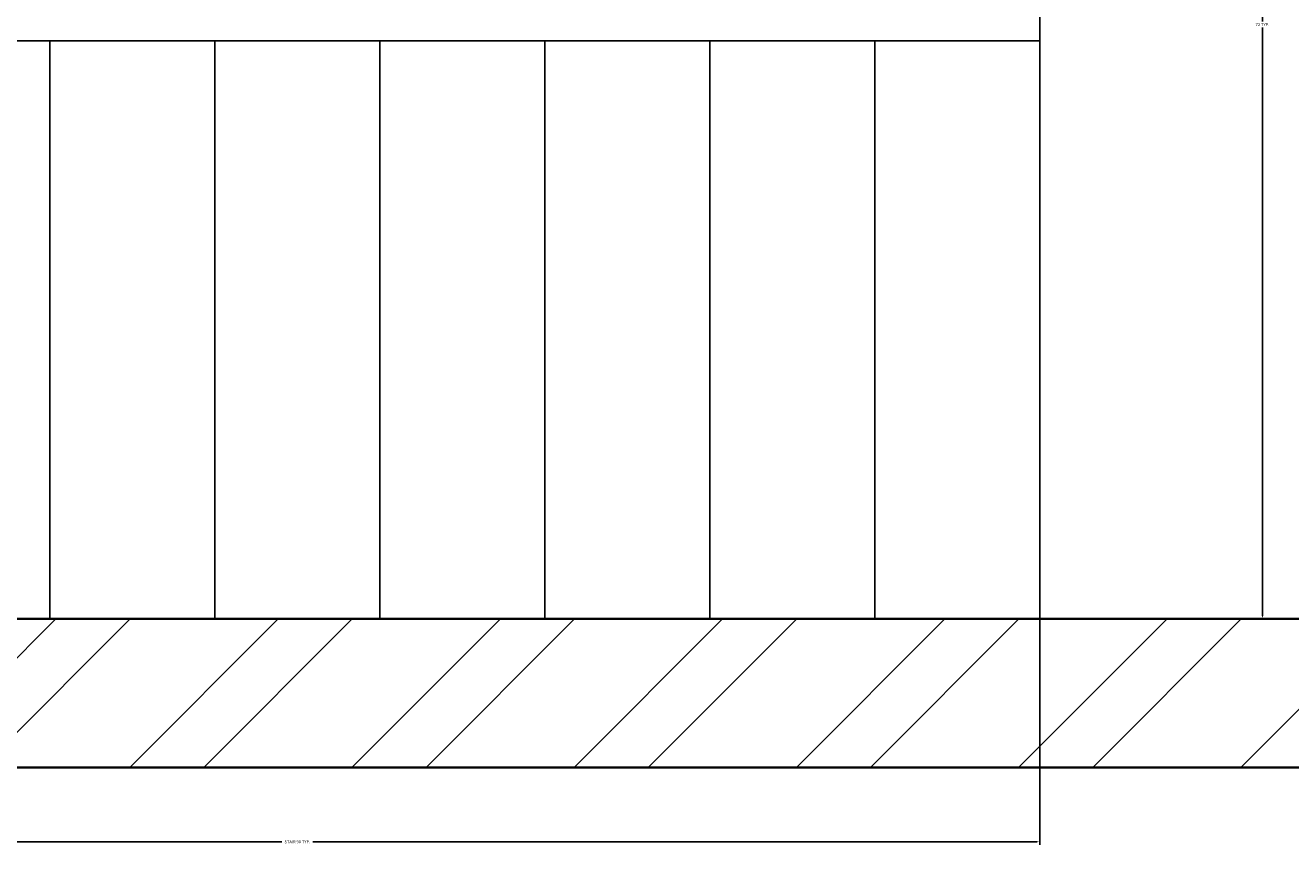
# Model space of a CAD drawing. Units: inches. Extents: x 2166 to 3588, y 1959 to 2628.
# Tile 9 of 13: x 3457 to 3534, y 2017 to 2067. Entities that reach past the tile are written whole.
import ezdxf

# ---------------------------------------------------------------- set-up
doc = ezdxf.new("R2010")
doc.units = ezdxf.units.IN
for name, color, linetype, lineweight in [('A-ANNO-DIMS', 2, 'Continuous', 18), ('A-AREA-IDEN', 170, 'Continuous', 18), ('A-WALL-PATT', 20, 'Continuous', 13), ('Staircase', 136, 'Continuous', 25), ('WALL', 40, 'Continuous', 35)]:
    doc.layers.add(name, color=color, linetype=linetype, lineweight=lineweight)
doc.styles.get("Standard").update_dxf_attribs({"font": 'arial.ttf'})
doc.dimstyles.get("Standard").update_dxf_attribs({"dimtxt": 0.18, "dimasz": 0.18, "dimexe": 0.18, "dimexo": 0.0625, "dimgap": 0.09, "dimtad": 0, "dimtih": 1, "dimtoh": 1, "dimdec": 4, "dimzin": 0, "dimdsep": 46, "dimtxsty": 'Standard', "dimcen": 0.09, "dimadec": 0, "dimazin": 0, "dimtfac": 1, "dimtdec": 4, "dimtofl": 0, "dimtmove": 0, "dimatfit": 3, "dimfxl": 1, "dimtolj": 1, "dimtzin": 0, "dimarcsym": 0})

# ---------------------------------------------------------------- blocks, each defined once
blk = doc.blocks.new('STAIR-RETURN-FLIGHTS')
for p, q in [((90, 72), (90, 0)), ((90, 35), (0, 35)), ((30, 35), (30, 0)), ((40, 35), (40, 0)), ((50, 35), (50, 0)), ((60, 35), (60, 0)), ((70, 35), (70, 0)), ((80, 35), (80, 0))]:
    blk.add_line(p, q)
blk = doc.blocks.new('*D17')
at = {"layer": 'A-ANNO-DIMS', "color": 0, "lineweight": -2, "transparency": 16777216}
for p, q in [((3428.471, 2030.916), (3428.471, 2017.299)), ((3518.471, 2030.916), (3518.471, 2017.299)), ((3428.651, 2017.479), (3472.538, 2017.479)), ((3518.291, 2017.479), (3474.403, 2017.479))]:
    blk.add_line(p, q, dxfattribs=at)
at = {"layer": 'A-ANNO-DIMS', "color": 0, "transparency": 16777216}
for points in [[(3428.651, 2017.509), (3428.651, 2017.449), (3428.471, 2017.479)], [(3518.291, 2017.509), (3518.291, 2017.449), (3518.471, 2017.479)]]:
    blk.add_solid(points, dxfattribs=at)
at = {"layer": 'Defpoints', "color": 0, "transparency": 16777216}
for p in [(3428.471, 2030.979), (3518.471, 2030.979), (3518.471, 2017.479)]:
    blk.add_point(p, dxfattribs=at)
at = {"layer": 'A-ANNO-DIMS', "color": 0, "transparency": 16777216, "insert": (3473.471, 2017.479), "char_height": 0.18, "attachment_point": 5}
blk.add_mtext('\\A1;STAIR 90 TYP.', dxfattribs=at)
blk = doc.blocks.new('*D18')
at = {"layer": 'A-ANNO-DIMS', "color": 0, "lineweight": -2, "transparency": 16777216}
for p, q in [((3518.533, 2102.979), (3532.151, 2102.979)), ((3531.971, 2102.799), (3531.971, 2067.159)), ((3531.971, 2031.159), (3531.971, 2066.799)), ((3518.533, 2030.979), (3532.151, 2030.979))]:
    blk.add_line(p, q, dxfattribs=at)
at = {"layer": 'A-ANNO-DIMS', "color": 0, "transparency": 16777216}
for points in [[(3531.941, 2102.799), (3532.001, 2102.799), (3531.971, 2102.979)], [(3531.941, 2031.159), (3532.001, 2031.159), (3531.971, 2030.979)]]:
    blk.add_solid(points, dxfattribs=at)
at = {"layer": 'Defpoints', "color": 0, "transparency": 16777216}
for p in [(3518.471, 2102.979), (3531.971, 2102.979), (3518.471, 2030.979)]:
    blk.add_point(p, dxfattribs=at)
at = {"layer": 'A-ANNO-DIMS', "color": 0, "transparency": 16777216, "insert": (3531.971, 2066.979), "char_height": 0.18, "attachment_point": 5}
blk.add_mtext('\\A1;72 TYP.', dxfattribs=at)

msp = doc.modelspace()

# ---------------------------------------------------------------- hatches: boundary and pattern name
at = {"layer": 'A-WALL-PATT'}
h = msp.add_hatch(dxfattribs=at)
h.set_pattern_fill('ANSI32', color=256)
h.paths.add_polyline_path([(3563.471, 2429.979), (3227.471, 2429.979), (3227.471, 2021.979), (3563.471, 2021.979)])
h.paths.add_polyline_path([(3236.471, 2420.979), (3554.471, 2420.979), (3554.471, 2111.979), (3236.471, 2111.979)], flags=16)
h.paths.add_polyline_path([(3236.471, 2102.979), (3554.471, 2102.979), (3554.471, 2030.979), (3236.471, 2030.979)], flags=16)
h.paths.add_polyline_path([(3518.471, 2085.283), (3518.471, 2067.979), (3458.471, 2067.979), (3458.471, 2085.283)], flags=0)
h.paths.add_polyline_path([(3434.656, 2082.283), (3442.194, 2082.283), (3442.194, 2087.514), (3434.656, 2087.514)], flags=8)
h.paths.add_polyline_path([(3522.671, 2094.512), (3521.752, 2052.984), (3545.541, 2052.457), (3546.46, 2093.986)], flags=8)

# ---------------------------------------------------------------- linework, layer by layer
at = {"layer": 'WALL'}
msp.add_lwpolyline([(3227.471, 2429.979), (3563.471, 2429.979), (3563.471, 2021.979), (3227.471, 2021.979)], close=True, dxfattribs=at)
msp.add_lwpolyline([(3554.471, 2102.979), (3554.471, 2030.979), (3236.471, 2030.979), (3236.471, 2102.979)], dxfattribs=at)

# ---------------------------------------------------------------- block references
at = {"layer": 'Staircase'}
msp.add_blockref('STAIR-RETURN-FLIGHTS', (3428.471, 2030.979), dxfattribs=at)

# ---------------------------------------------------------------- texts
at = {"layer": 'A-AREA-IDEN', "insert": (3545.955, 2091.996), "char_height": 8, "attachment_point": 1, "rotation": 268.73191}
msp.add_mtext_dynamic_manual_height_columns("{\\Fsuperos|c0;LANDING\\P   3'}", width=58.85395, gutter_width=12.5, heights=[0], dxfattribs=at)

# ---------------------------------------------------------------- dimensions: what is measured, and where the dimension line sits
at = {"layer": 'A-ANNO-DIMS'}
dim = msp.add_linear_dim(base=(3531.971, 2102.979), p1=(3518.471, 2030.979), p2=(3518.471, 2102.979), angle=90, text='<> TYP.', dimstyle='Standard', override={"dimdec": 0, "dimlfac": 1, "dimrnd": 0, "dimzin": 0, "dimdsep": 46, "dimlunit": 2}, dxfattribs=at)
dim.commit()
dim.dimension.update_dxf_attribs({"geometry": '*D18', "text_midpoint": (3531.971, 2066.979)})
dim = msp.add_linear_dim(base=(3518.471, 2017.479), p1=(3428.471, 2030.979), p2=(3518.471, 2030.979), text='STAIR <> TYP.', dimstyle='Standard', override={"dimdec": 0, "dimlfac": 1, "dimrnd": 0, "dimzin": 0, "dimdsep": 46, "dimlunit": 2}, dxfattribs=at)
dim.commit()
dim.dimension.update_dxf_attribs({"geometry": '*D17', "text_midpoint": (3473.471, 2017.479)})

doc.saveas('drawing.dxf')
